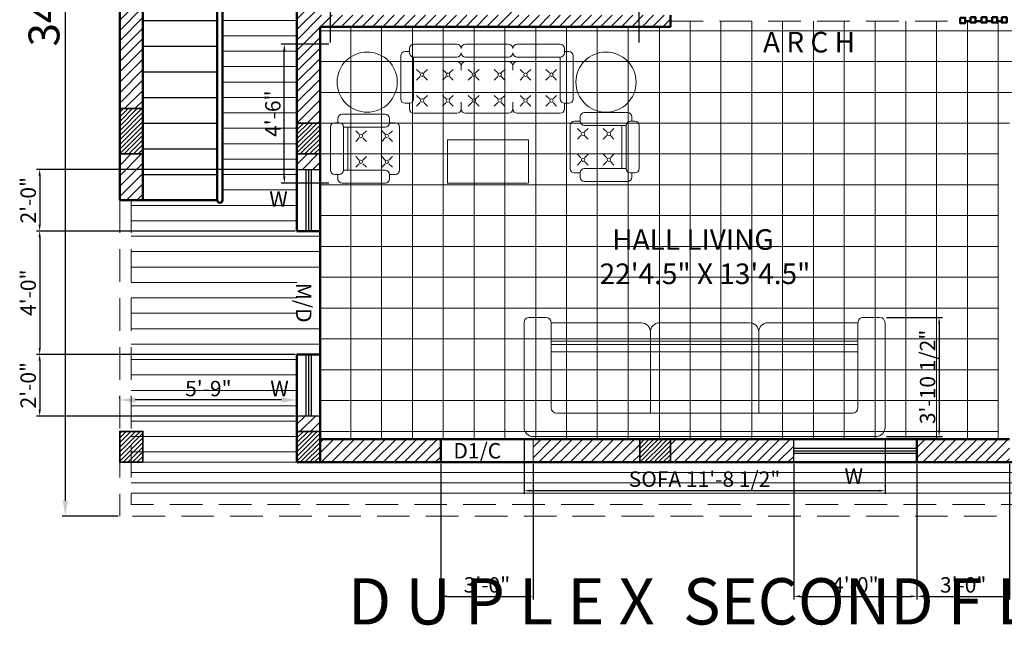
# Model space of a CAD drawing. Units: millimetres. Extents: x 225995 to 227247, y 225507 to 226008.
# Tile 1 of 23: x 225995 to 226378, y 225507 to 225743. Entities that reach past the tile are written whole.
import ezdxf

# ---------------------------------------------------------------- set-up
doc = ezdxf.new("R2010")
doc.units = ezdxf.units.MM
doc.linetypes.add('DASHED', pattern=[19.05, 12.7, -6.35])
for name, color, linetype, lineweight in [('A-ANNO-DIMS', 2, 'Continuous', 18), ('A-ANNO-TEXT', 3, 'Continuous', 18), ('A-AREA-IDEN', 30, 'Continuous', 18), ('A-COLS', 40, 'Continuous', 35), ('A-FLOR-PATT', 8, 'Continuous', 13), ('A-FLOR-STRS', 141, 'Continuous', 25), ('A-FURN', 9, 'Continuous', 18), ('A-GLAZ', 4, 'Continuous', 25), ('A-WALL', 7, 'Continuous', 50), ('A-WALL-OVHD', 1, 'DASHED', 18), ('A-WALL-PATT', 8, 'Continuous', 13)]:
    doc.layers.add(name, color=color, linetype=linetype, lineweight=lineweight)
doc.styles.get("Standard").update_dxf_attribs({"font": 'arial.ttf'})
doc.dimstyles.new('ISO-25', dxfattribs={"dimtxt": 6, "dimasz": 2.5, "dimexe": 1.25, "dimexo": 0.625, "dimtad": 1, "dimdec": 0, "dimlunit": 3, "dimtxsty": 'Standard', "dimcen": 2.5, "dimadec": 0, "dimazin": 0, "dimtfac": 1, "dimtdec": 0, "dimtmove": 0, "dimatfit": 3, "dimfxl": 1, "dimarcsym": 0})
pattern_1 = [(45, (-144, -120), (-0.898025612, 0.898025612), [])]

# ---------------------------------------------------------------- blocks, each defined once
blk = doc.blocks.new('A$C144B2C1F')
at = {"linetype": 'ByBlock'}
for p, q in [((1465, 1610), (965, 1610)), ((2065, 1610), (1565, 1610)), ((2665, 1610), (2165, 1610)), ((914, 1526), (864, 1526)), ((915, 1560), (915, 1510)), ((2764, 1526), (2714, 1526)), ((2715, 1510), (2715, 1560)), ((814, 1476), (814, 976)), ((964, 976), (964, 1460)), ((965, 1460), (1465, 1460)), ((965, 1410), (1465, 1410)), ((1565, 1460), (2065, 1460)), ((1565, 1410), (2065, 1410)), ((2165, 1460), (2665, 1460)), ((2165, 1410), (2664, 1410)), ((2664, 1460), (2664, 976)), ((2814, 976), (2814, 1476)), ((1040, 1277), (998, 1317)), ((1081, 1277), (1123, 1317)), ((1340, 1277), (1298, 1317)), ((1381, 1277), (1423, 1317)), ((1515, 1311), (1515, 1360)), ((1640, 1277), (1598, 1317)), ((1681, 1277), (1723, 1317)), ((1940, 1277), (1898, 1317)), ((1981, 1277), (2023, 1317)), ((2115, 1311), (2115, 1360)), ((2240, 1277), (2198, 1317)), ((2281, 1277), (2323, 1317)), ((2540, 1277), (2498, 1317)), ((2581, 1277), (2623, 1317)), ((1040, 1235), (998, 1193)), ((1081, 1235), (1123, 1193)), ((1340, 1235), (1298, 1193)), ((1381, 1235), (1423, 1193)), ((1640, 1235), (1598, 1193)), ((1681, 1235), (1723, 1193)), ((1940, 1235), (1898, 1193)), ((1981, 1235), (2023, 1193)), ((2240, 1235), (2198, 1193)), ((2281, 1235), (2323, 1193)), ((2540, 1235), (2498, 1193)), ((2581, 1235), (2623, 1193)), ((864, 926), (914, 926)), ((915, 926), (915, 860)), ((1040, 977), (998, 1017)), ((1040, 935), (998, 893)), ((1081, 977), (1123, 1017)), ((1081, 935), (1123, 893)), ((1340, 977), (1298, 1017)), ((1340, 935), (1298, 893)), ((1381, 977), (1423, 1017)), ((1381, 935), (1423, 893)), ((1515, 860), (1515, 937)), ((1515, 926), (1515, 860)), ((1640, 977), (1598, 1017)), ((1640, 935), (1598, 893)), ((1681, 977), (1723, 1017)), ((1681, 935), (1723, 893)), ((1940, 977), (1898, 1017)), ((1940, 935), (1898, 893)), ((1981, 977), (2023, 1017)), ((1981, 935), (2023, 893)), ((2115, 860), (2115, 937)), ((2115, 926), (2115, 860)), ((2240, 977), (2198, 1017)), ((2240, 935), (2198, 893)), ((2281, 977), (2323, 1017)), ((2281, 935), (2323, 893)), ((2540, 977), (2498, 1017)), ((2540, 935), (2498, 893)), ((2581, 977), (2623, 1017)), ((2581, 935), (2623, 893)), ((2714, 926), (2764, 926)), ((2715, 860), (2715, 926)), ((634, 800), (134, 800)), ((1129, 810), (965, 810)), ((1465, 810), (1088, 810)), ((1729, 810), (1565, 810)), ((2065, 810), (1688, 810)), ((2329, 810), (2165, 810)), ((2665, 810), (2288, 810)), ((3446, 819), (2946, 819)), ((100, 701), (50, 701)), ((84, 750), (84, 700)), ((684, 700), (684, 750)), ((750, 701), (684, 701)), ((2896, 718), (2830, 718)), ((2896, 769), (2896, 719)), ((3530, 718), (3480, 718)), ((3496, 719), (3496, 769)), ((0, 651), (0, 151)), ((150, 151), (150, 651)), ((150, 650), (634, 650)), ((200, 151), (200, 650)), ((333, 567), (293, 608)), ((375, 567), (418, 608)), ((633, 567), (593, 608)), ((675, 567), (718, 608)), ((800, 651), (800, 274)), ((2780, 504), (2780, 668)), ((2905, 593), (2863, 635)), ((2946, 669), (3430, 669)), ((2948, 593), (2987, 635)), ((3205, 593), (3163, 635)), ((3248, 593), (3287, 635)), ((3380, 668), (3380, 169)), ((3430, 668), (3430, 168)), ((3580, 168), (3580, 668)), ((333, 525), (293, 484)), ((375, 525), (418, 484)), ((633, 525), (593, 484)), ((675, 525), (718, 484)), ((2295, 501), (1355, 501)), ((1355, 501), (1355, 1)), ((2295, 1), (2295, 501)), ((2780, 168), (2780, 545)), ((2905, 552), (2863, 510)), ((2948, 552), (2987, 510)), ((3205, 552), (3163, 510)), ((3248, 552), (3287, 510)), ((333, 267), (293, 308)), ((375, 267), (418, 308)), ((633, 267), (593, 308)), ((675, 267), (718, 308)), ((800, 314), (800, 151)), ((2905, 293), (2863, 335)), ((2905, 252), (2863, 210)), ((2948, 293), (2987, 335)), ((2948, 252), (2987, 210)), ((3205, 293), (3163, 335)), ((3205, 252), (3163, 210)), ((3248, 293), (3287, 335)), ((3248, 252), (3287, 210)), ((634, 150), (150, 150)), ((333, 225), (293, 184)), ((375, 225), (418, 184)), ((633, 225), (593, 184)), ((675, 225), (718, 184)), ((2830, 118), (2896, 118)), ((2896, 119), (2896, 69)), ((3430, 169), (2946, 169)), ((3480, 118), (3530, 118)), ((3496, 69), (3496, 119)), ((50, 101), (100, 101)), ((84, 100), (84, 50)), ((134, 0), (634, 0)), ((684, 101), (750, 101)), ((684, 50), (684, 100)), ((1355, 1), (2285, 1)), ((2946, 19), (3446, 19))]:
    blk.add_line(p, q, dxfattribs=at)
for centre, radius in [((425, 1171), 349), ((3195, 1171), 349), ((1062, 1258), 20), ((1362, 1258), 20), ((1662, 1258), 20), ((1962, 1258), 20), ((2262, 1258), 20), ((2562, 1258), 20), ((1062, 958), 20), ((1362, 958), 20), ((1662, 958), 20), ((1962, 958), 20), ((2262, 958), 20), ((2562, 958), 20), ((2928, 571), 20), ((3228, 571), 20), ((352, 548), 20), ((652, 548), 20), ((352, 248), 20), ((652, 248), 20), ((2928, 271), 20), ((3228, 271), 20)]:
    blk.add_circle(centre, radius, dxfattribs=at)
for centre, start, end in [((965, 1560), 90, 180), ((965, 1560), 90, 180), ((1465, 1560), 0, 90), ((1565, 1560), 90, 180), ((1565, 1560), 90, 180), ((2065, 1560), 0, 90), ((2165, 1560), 90, 180), ((2165, 1560), 90, 180), ((2665, 1560), 0, 90), ((864, 1476), 90, 180), ((965, 1510), 180, 270), ((1465, 1510), 270, 0), ((1565, 1510), 180, 270), ((2065, 1510), 270, 0), ((2165, 1510), 180, 270), ((2665, 1510), 270, 0), ((2764, 1476), 0, 90), ((1465, 1360), 0, 90), ((1565, 1360), 90, 180), ((2065, 1360), 0, 90), ((2165, 1360), 90, 180), ((864, 976), 180, 270), ((914, 976), 270, 0), ((2714, 976), 180, 270), ((2764, 976), 270, 0), ((134, 750), 90, 180), ((634, 750), 0, 90), ((965, 860), 180, 270), ((1465, 860), 270, 0), ((1565, 860), 180, 270), ((2065, 860), 270, 0), ((2165, 860), 180, 270), ((2665, 860), 270, 0), ((2946, 769), 90, 180), ((3446, 769), 0, 90), ((50, 651), 90, 180), ((100, 651), 0, 90), ((634, 700), 270, 0), ((750, 651), 0, 90), ((2830, 668), 90, 180), ((2946, 719), 180, 270), ((3480, 668), 90, 180), ((3530, 668), 0, 90), ((3530, 668), 0, 90), ((50, 151), 180, 270), ((50, 151), 180, 270), ((100, 151), 270, 0), ((634, 100), 0, 90), ((750, 151), 270, 0), ((2830, 168), 180, 270), ((2946, 119), 90, 180), ((3480, 168), 180, 270), ((3530, 168), 270, 0), ((134, 50), 180, 270), ((634, 50), 270, 0), ((2946, 69), 180, 270), ((3446, 69), 270, 0)]:
    blk.add_arc(centre, 50, start, end, dxfattribs=at)
blk = doc.blocks.new('A$C05BA3A2B')
for p, q in [((0.05, 0.6596), (1.95, 0.6596)), ((0.05, 0.6596), (1.95, 0.6596)), ((0.05, 0.6596), (1.95, 0.6596)), ((0, 0.03), (0, 0.6096)), ((0, 0.03), (0, 0.6096)), ((0, 0.03), (0, 0.6096)), ((2, 0.6096), (2, 0.03)), ((2, 0.6096), (2, 0.03)), ((2, 0.6096), (2, 0.03)), ((0.15, 0.5), (0.15, 0.03)), ((0.15, 0.5), (0.15, 0.03)), ((0.15, 0.5), (0.15, 0.03)), ((1.82, 0.53), (0.18, 0.53)), ((1.82, 0.53), (0.18, 0.53)), ((1.82, 0.53), (0.18, 0.53)), ((0.7, 0.08), (0.7, 0.53)), ((0.7, 0.08), (0.7, 0.53)), ((0.7, 0.08), (0.7, 0.53)), ((1.3, 0.53), (1.3, 0.08)), ((1.3, 0.53), (1.3, 0.08)), ((1.3, 0.53), (1.3, 0.08)), ((1.85, 0.03), (1.85, 0.5)), ((1.85, 0.03), (1.85, 0.5)), ((1.85, 0.03), (1.85, 0.5)), ((1.85, 0.1908), (0.15, 0.1908)), ((1.85, 0.1908), (0.15, 0.1908)), ((1.85, 0.1908), (0.15, 0.1908)), ((1.85, 0.1508), (0.15, 0.1508)), ((1.85, 0.1508), (0.15, 0.1508)), ((1.85, 0.1508), (0.15, 0.1508)), ((1.85, 0.1308), (0.15, 0.1308)), ((1.85, 0.1308), (0.15, 0.1308)), ((1.85, 0.1308), (0.15, 0.1308)), ((0.12, 0), (0.03, 0)), ((0.12, 0), (0.03, 0)), ((0.12, 0), (0.03, 0)), ((0.65, 0.03), (0.15, 0.03)), ((0.65, 0.03), (0.15, 0.03)), ((0.65, 0.03), (0.15, 0.03)), ((1.25, 0.03), (0.75, 0.03)), ((1.25, 0.03), (0.75, 0.03)), ((1.25, 0.03), (0.75, 0.03)), ((1.85, 0.03), (1.35, 0.03)), ((1.85, 0.03), (1.35, 0.03)), ((1.85, 0.03), (1.35, 0.03)), ((1.97, 0), (1.88, 0)), ((1.97, 0), (1.88, 0)), ((1.97, 0), (1.88, 0))]:
    blk.add_line(p, q)
for centre, radius, start, end in [((0.05, 0.6096), 0.05, 90, 180), ((0.05, 0.6096), 0.05, 90, 180), ((0.05, 0.6096), 0.05, 90, 180), ((1.95, 0.6096), 0.05, 0, 90), ((1.95, 0.6096), 0.05, 0, 90), ((1.95, 0.6096), 0.05, 0, 90), ((0.18, 0.5), 0.03, 90, 180), ((0.18, 0.5), 0.03, 90, 180), ((0.18, 0.5), 0.03, 90, 180), ((1.82, 0.5), 0.03, 0, 90), ((1.82, 0.5), 0.03, 0, 90), ((1.82, 0.5), 0.03, 0, 90), ((0.65, 0.08), 0.05, 270, 0), ((0.65, 0.08), 0.05, 270, 0), ((0.65, 0.08), 0.05, 270, 0), ((0.75, 0.08), 0.05, 180, 270), ((0.75, 0.08), 0.05, 180, 270), ((0.75, 0.08), 0.05, 180, 270), ((1.25, 0.08), 0.05, 270, 0), ((1.25, 0.08), 0.05, 270, 0), ((1.25, 0.08), 0.05, 270, 0), ((1.35, 0.08), 0.05, 180, 270), ((1.35, 0.08), 0.05, 180, 270), ((1.35, 0.08), 0.05, 180, 270), ((0.03, 0.03), 0.03, 180, 270), ((0.03, 0.03), 0.03, 180, 270), ((0.03, 0.03), 0.03, 180, 270), ((0.12, 0.03), 0.03, 270, 0), ((0.12, 0.03), 0.03, 270, 0), ((0.12, 0.03), 0.03, 270, 0), ((1.88, 0.03), 0.03, 180, 270), ((1.88, 0.03), 0.03, 180, 270), ((1.88, 0.03), 0.03, 180, 270), ((1.97, 0.03), 0.03, 270, 0), ((1.97, 0.03), 0.03, 270, 0), ((1.97, 0.03), 0.03, 270, 0)]:
    blk.add_arc(centre, radius, start, end)
blk = doc.blocks.new('A$C720744B6')
blk.add_blockref('A$C05BA3A2B', (0, 0))
blk = doc.blocks.new('*D66')
at = {"layer": 'A-ANNO-DIMS', "color": 0, "lineweight": -2, "transparency": 16777216}
for p, q in [((226033.88, 225595.63), (226033.88, 225596.26)), ((226096.88, 225595.01), (226039.88, 225595.01)), ((226102.88, 225595.63), (226102.88, 225596.26))]:
    blk.add_line(p, q, dxfattribs=at)
at = {"layer": 'A-ANNO-DIMS', "color": 0, "transparency": 16777216}
for points in [[(226039.88, 225596.01), (226039.88, 225594.01), (226033.88, 225595.01)], [(226096.88, 225596.01), (226096.88, 225594.01), (226102.88, 225595.01)]]:
    blk.add_solid(points, dxfattribs=at)
at = {"layer": 'Defpoints', "color": 0, "transparency": 16777216}
for p in [(226033.88, 225595.01), (226033.88, 225595.01), (226102.88, 225595.01)]:
    blk.add_point(p, dxfattribs=at)
at = {"layer": 'A-ANNO-DIMS', "color": 0, "transparency": 16777216, "insert": (226068.38, 225598.69), "char_height": 6, "attachment_point": 5}
blk.add_mtext('5\'-9"', dxfattribs=at)
blk = doc.blocks.new('*D69')
at = {"layer": 'A-ANNO-DIMS', "color": 0, "lineweight": -2, "transparency": 16777216}
for p, q in [((226033.25, 225960.77), (226011.42, 225960.77)), ((226012.67, 225954.77), (226012.67, 225555.77)), ((226033.25, 225549.77), (226011.42, 225549.77))]:
    blk.add_line(p, q, dxfattribs=at)
at = {"layer": 'A-ANNO-DIMS', "color": 0, "transparency": 16777216}
for points in [[(226011.67, 225954.77), (226013.67, 225954.77), (226012.67, 225960.77)], [(226011.67, 225555.77), (226013.67, 225555.77), (226012.67, 225549.77)]]:
    blk.add_solid(points, dxfattribs=at)
at = {"layer": 'Defpoints', "color": 0, "transparency": 16777216}
for p in [(226033.88, 225960.77), (226012.67, 225549.77), (226033.88, 225549.77)]:
    blk.add_point(p, dxfattribs=at)
at = {"layer": 'A-ANNO-DIMS', "color": 0, "transparency": 16777216, "insert": (226005.92, 225755.27), "char_height": 12, "attachment_point": 5, "rotation": 90}
blk.add_mtext('34\'-3"', dxfattribs=at)
blk = doc.blocks.new('*D83')
at = {"layer": 'A-ANNO-DIMS', "color": 0, "lineweight": -2, "transparency": 16777216}
for p, q in [((226115.99, 225734.11), (226115.99, 225752.77)), ((226118.49, 225751.52), (226233.69, 225751.52)), ((226236.19, 225734.11), (226236.19, 225752.77))]:
    blk.add_line(p, q, dxfattribs=at)
at = {"layer": 'A-ANNO-DIMS', "color": 0, "transparency": 16777216}
for points in [[(226118.49, 225751.93), (226118.49, 225751.1), (226115.99, 225751.52)], [(226233.69, 225751.93), (226233.69, 225751.1), (226236.19, 225751.52)]]:
    blk.add_solid(points, dxfattribs=at)
at = {"layer": 'Defpoints', "color": 0, "transparency": 16777216}
for p in [(226236.19, 225751.52), (226115.99, 225733.49), (226236.19, 225733.49)]:
    blk.add_point(p, dxfattribs=at)
at = {"layer": 'A-ANNO-DIMS', "color": 0, "transparency": 16777216, "insert": (226176.09, 225755.25), "char_height": 6, "attachment_point": 5}
blk.add_mtext('SOFA SET 10\'-0"', dxfattribs=at)
blk = doc.blocks.new('*D84')
at = {"layer": 'A-ANNO-DIMS', "color": 0, "lineweight": -2, "transparency": 16777216}
for p, q in [((226115.37, 225733.49), (226096.71, 225733.49)), ((226097.96, 225681.93), (226097.96, 225730.99)), ((226115.37, 225679.43), (226096.71, 225679.43))]:
    blk.add_line(p, q, dxfattribs=at)
at = {"layer": 'A-ANNO-DIMS', "color": 0, "transparency": 16777216}
for points in [[(226097.54, 225730.99), (226098.38, 225730.99), (226097.96, 225733.49)], [(226097.54, 225681.93), (226098.38, 225681.93), (226097.96, 225679.43)]]:
    blk.add_solid(points, dxfattribs=at)
at = {"layer": 'Defpoints', "color": 0, "transparency": 16777216}
for p in [(226097.96, 225733.49), (226115.99, 225733.49), (226115.99, 225679.43)]:
    blk.add_point(p, dxfattribs=at)
at = {"layer": 'A-ANNO-DIMS', "color": 0, "transparency": 16777216, "insert": (226094.27, 225706.46), "char_height": 6, "attachment_point": 5, "rotation": 90}
blk.add_mtext('4\'-6"', dxfattribs=at)
blk = doc.blocks.new('*D85')
at = {"layer": 'A-ANNO-DIMS', "color": 0, "lineweight": -2, "transparency": 16777216}
for p, q in [((226191.34, 225580.17), (226191.34, 225558.45)), ((226331.94, 225580.17), (226331.94, 225558.45)), ((226329.44, 225559.7), (226193.84, 225559.7))]:
    blk.add_line(p, q, dxfattribs=at)
at = {"layer": 'A-ANNO-DIMS', "color": 0, "transparency": 16777216}
for points in [[(226193.84, 225560.12), (226193.84, 225559.29), (226191.34, 225559.7)], [(226329.44, 225560.12), (226329.44, 225559.29), (226331.94, 225559.7)]]:
    blk.add_solid(points, dxfattribs=at)
at = {"layer": 'Defpoints', "color": 0, "transparency": 16777216}
for p in [(226191.34, 225580.79), (226331.94, 225580.79), (226191.34, 225559.7)]:
    blk.add_point(p, dxfattribs=at)
at = {"layer": 'A-ANNO-DIMS', "color": 0, "transparency": 16777216, "insert": (226261.64, 225563.43), "char_height": 6, "attachment_point": 5}
blk.add_mtext('SOFA 11\'-8 1/2"', dxfattribs=at)
blk = doc.blocks.new('*D86')
at = {"layer": 'A-ANNO-DIMS', "color": 0, "lineweight": -2, "transparency": 16777216}
for p, q in [((226332.56, 225627.16), (226354.27, 225627.16)), ((226353.02, 225624.66), (226353.02, 225583.29)), ((226332.56, 225580.79), (226354.27, 225580.79))]:
    blk.add_line(p, q, dxfattribs=at)
at = {"layer": 'A-ANNO-DIMS', "color": 0, "transparency": 16777216}
for points in [[(226352.61, 225624.66), (226353.44, 225624.66), (226353.02, 225627.16)], [(226352.61, 225583.29), (226353.44, 225583.29), (226353.02, 225580.79)]]:
    blk.add_solid(points, dxfattribs=at)
at = {"layer": 'Defpoints', "color": 0, "transparency": 16777216}
for p in [(226331.94, 225627.16), (226331.94, 225580.79), (226353.02, 225580.79)]:
    blk.add_point(p, dxfattribs=at)
at = {"layer": 'A-ANNO-DIMS', "color": 0, "transparency": 16777216, "insert": (226349.3, 225603.98), "char_height": 6, "attachment_point": 5, "rotation": 90}
blk.add_mtext('3\'-10 1/2"', dxfattribs=at)
blk = doc.blocks.new('*D106')
at = {"layer": 'A-ANNO-DIMS', "color": 0, "lineweight": -2, "transparency": 16777216}
for p, q in [((226296.38, 225570.15), (226296.38, 225517.32)), ((226344.38, 225570.15), (226344.38, 225517.32)), ((226298.88, 225518.57), (226341.88, 225518.57))]:
    blk.add_line(p, q, dxfattribs=at)
at = {"layer": 'A-ANNO-DIMS', "color": 0, "transparency": 16777216}
for points in [[(226298.88, 225518.99), (226298.88, 225518.16), (226296.38, 225518.57)], [(226341.88, 225518.99), (226341.88, 225518.16), (226344.38, 225518.57)]]:
    blk.add_solid(points, dxfattribs=at)
at = {"layer": 'Defpoints', "color": 0, "transparency": 16777216}
for p in [(226296.38, 225570.77), (226344.38, 225570.77), (226344.38, 225518.57)]:
    blk.add_point(p, dxfattribs=at)
at = {"layer": 'A-ANNO-DIMS', "color": 0, "transparency": 16777216, "insert": (226320.38, 225522.26), "char_height": 6, "attachment_point": 5}
blk.add_mtext('4\'-0"', dxfattribs=at)
blk = doc.blocks.new('*D107')
at = {"layer": 'A-ANNO-DIMS', "color": 0, "lineweight": -2, "transparency": 16777216}
for p, q in [((226344.38, 225570.15), (226344.38, 225517.32)), ((226380.38, 225570.15), (226380.38, 225517.32)), ((226346.88, 225518.57), (226377.88, 225518.57))]:
    blk.add_line(p, q, dxfattribs=at)
at = {"layer": 'A-ANNO-DIMS', "color": 0, "transparency": 16777216}
for points in [[(226346.88, 225518.99), (226346.88, 225518.16), (226344.38, 225518.57)], [(226377.88, 225518.99), (226377.88, 225518.16), (226380.38, 225518.57)]]:
    blk.add_solid(points, dxfattribs=at)
at = {"layer": 'Defpoints', "color": 0, "transparency": 16777216}
for p in [(226344.38, 225570.77), (226380.38, 225570.77), (226380.38, 225518.57)]:
    blk.add_point(p, dxfattribs=at)
at = {"layer": 'A-ANNO-DIMS', "color": 0, "transparency": 16777216, "insert": (226362.38, 225522.26), "char_height": 6, "attachment_point": 5}
blk.add_mtext('3\'-0"', dxfattribs=at)
blk = doc.blocks.new('*D108')
at = {"layer": 'A-ANNO-DIMS', "color": 0, "lineweight": -2, "transparency": 16777216}
for p, q in [((226158.88, 225570.15), (226158.88, 225517.32)), ((226194.88, 225570.15), (226194.88, 225517.32)), ((226161.38, 225518.57), (226192.38, 225518.57))]:
    blk.add_line(p, q, dxfattribs=at)
at = {"layer": 'A-ANNO-DIMS', "color": 0, "transparency": 16777216}
for points in [[(226161.38, 225518.99), (226161.38, 225518.16), (226158.88, 225518.57)], [(226192.38, 225518.99), (226192.38, 225518.16), (226194.88, 225518.57)]]:
    blk.add_solid(points, dxfattribs=at)
at = {"layer": 'Defpoints', "color": 0, "transparency": 16777216}
for p in [(226158.88, 225570.77), (226194.88, 225570.77), (226194.88, 225518.57)]:
    blk.add_point(p, dxfattribs=at)
at = {"layer": 'A-ANNO-DIMS', "color": 0, "transparency": 16777216, "insert": (226176.88, 225522.26), "char_height": 6, "attachment_point": 5}
blk.add_mtext('3\'-0"', dxfattribs=at)
blk = doc.blocks.new('*D109')
at = {"layer": 'A-ANNO-DIMS', "color": 0, "lineweight": -2, "transparency": 16777216}
for p, q in [((226102.25, 225684.77), (226001.43, 225684.77)), ((226002.68, 225682.27), (226002.68, 225663.27)), ((226102.25, 225660.77), (226001.43, 225660.77))]:
    blk.add_line(p, q, dxfattribs=at)
at = {"layer": 'A-ANNO-DIMS', "color": 0, "transparency": 16777216}
for points in [[(226002.26, 225682.27), (226003.09, 225682.27), (226002.68, 225684.77)], [(226002.26, 225663.27), (226003.09, 225663.27), (226002.68, 225660.77)]]:
    blk.add_solid(points, dxfattribs=at)
at = {"layer": 'Defpoints', "color": 0, "transparency": 16777216}
for p in [(226102.88, 225684.77), (226002.68, 225660.77), (226102.88, 225660.77)]:
    blk.add_point(p, dxfattribs=at)
at = {"layer": 'A-ANNO-DIMS', "color": 0, "transparency": 16777216, "insert": (225998.99, 225672.77), "char_height": 6, "attachment_point": 5, "rotation": 90}
blk.add_mtext('2\'-0"', dxfattribs=at)
blk = doc.blocks.new('*D110')
at = {"layer": 'A-ANNO-DIMS', "color": 0, "lineweight": -2, "transparency": 16777216}
for p, q in [((226102.25, 225660.77), (226001.43, 225660.77)), ((226002.68, 225658.27), (226002.68, 225615.27)), ((226102.25, 225612.77), (226001.43, 225612.77))]:
    blk.add_line(p, q, dxfattribs=at)
at = {"layer": 'A-ANNO-DIMS', "color": 0, "transparency": 16777216}
for points in [[(226002.26, 225658.27), (226003.09, 225658.27), (226002.68, 225660.77)], [(226002.26, 225615.27), (226003.09, 225615.27), (226002.68, 225612.77)]]:
    blk.add_solid(points, dxfattribs=at)
at = {"layer": 'Defpoints', "color": 0, "transparency": 16777216}
for p in [(226102.88, 225660.77), (226002.68, 225612.77), (226102.88, 225612.77)]:
    blk.add_point(p, dxfattribs=at)
at = {"layer": 'A-ANNO-DIMS', "color": 0, "transparency": 16777216, "insert": (225998.99, 225636.77), "char_height": 6, "attachment_point": 5, "rotation": 90}
blk.add_mtext('4\'-0"', dxfattribs=at)
blk = doc.blocks.new('*D111')
at = {"layer": 'A-ANNO-DIMS', "color": 0, "lineweight": -2, "transparency": 16777216}
for p, q in [((226102.25, 225612.77), (226001.43, 225612.77)), ((226002.68, 225610.27), (226002.68, 225591.27)), ((226102.25, 225588.77), (226001.43, 225588.77))]:
    blk.add_line(p, q, dxfattribs=at)
at = {"layer": 'A-ANNO-DIMS', "color": 0, "transparency": 16777216}
for points in [[(226002.26, 225610.27), (226003.09, 225610.27), (226002.68, 225612.77)], [(226002.26, 225591.27), (226003.09, 225591.27), (226002.68, 225588.77)]]:
    blk.add_solid(points, dxfattribs=at)
at = {"layer": 'Defpoints', "color": 0, "transparency": 16777216}
for p in [(226102.88, 225612.77), (226002.68, 225588.77), (226102.88, 225588.77)]:
    blk.add_point(p, dxfattribs=at)
at = {"layer": 'A-ANNO-DIMS', "color": 0, "transparency": 16777216, "insert": (225998.99, 225600.77), "char_height": 6, "attachment_point": 5, "rotation": 90}
blk.add_mtext('2\'-0"', dxfattribs=at)

msp = doc.modelspace()

# ---------------------------------------------------------------- hatches: boundary and pattern name
at = {"layer": 'A-WALL-PATT'}
h = msp.add_hatch(dxfattribs=at)
h.set_pattern_fill('ANSI31', color=256, scale=0.9)
h.paths.add_polyline_path([(226042.88, 225894.68), (226033.88, 225894.68), (226033.88, 225708.42), (226042.88, 225708.42)])
h = msp.add_hatch(dxfattribs=at)
h.set_pattern_fill('ANSI31', color=256, scale=0.9)
h.paths.add_polyline_path([(226111.88, 225740.27), (226248.38, 225740.27), (226248.38, 225744.77), (226188.38, 225744.77), (226188.38, 225756.77), (226183.88, 225756.77), (226183.88, 225744.77), (226111.88, 225744.77), (226111.88, 225762.77), (226102.88, 225762.77), (226102.88, 225702.77), (226111.88, 225702.77)])
h = msp.add_hatch(dxfattribs=at)
h.set_pattern_fill('ANSI31', color=256, scale=0.4)
h.paths.add_polyline_path([(226042.88, 225708.42), (226033.88, 225708.42), (226033.88, 225690.77), (226042.88, 225690.77)])
h = msp.add_hatch(dxfattribs=at)
h.set_pattern_fill('ANSI31', color=256, scale=0.4)
h.set_pattern_definition([(45, (-3e-11, 120), (-0.898025612, 0.898025612), [])])
h.paths.add_polyline_path([(226111.88, 225702.77), (226102.88, 225702.77), (226102.88, 225690.77), (226111.88, 225690.77)])
h = msp.add_hatch(dxfattribs=at)
h.set_pattern_fill('ANSI31', color=256, scale=0.9)
h.paths.add_polyline_path([(226042.88, 225690.77), (226033.88, 225690.77), (226033.88, 225672.77), (226042.88, 225672.77)])
h = msp.add_hatch(dxfattribs=at)
h.set_pattern_fill('ANSI31', color=256, scale=0.9)
h.paths.add_polyline_path([(226111.88, 225690.77), (226102.88, 225690.77), (226102.88, 225684.77), (226111.88, 225684.77)])
h = msp.add_hatch(dxfattribs=at)
h.set_pattern_fill('ANSI31', color=256, scale=0.9)
h.paths.add_polyline_path([(226111.88, 225588.77), (226102.88, 225588.77), (226102.88, 225582.77), (226111.88, 225582.77)])
h = msp.add_hatch(dxfattribs=at)
h.set_pattern_fill('ANSI31', color=256, scale=0.4)
h.set_pattern_definition([(45, (-69, 0), (-0.898025612, 0.898025612), [])])
h.paths.add_polyline_path([(226042.88, 225582.77), (226033.88, 225582.77), (226033.88, 225570.77), (226042.88, 225570.77)])
h = msp.add_hatch(dxfattribs=at)
h.set_pattern_fill('ANSI31', color=256, scale=0.4)
h.paths.add_polyline_path([(226111.88, 225582.77), (226102.88, 225582.77), (226102.88, 225570.77), (226111.88, 225570.77)])
h = msp.add_hatch(dxfattribs=at)
h.set_pattern_fill('ANSI31', color=256, scale=0.9)
h.paths.add_polyline_path([(226158.88, 225579.77), (226111.88, 225579.77), (226111.88, 225570.77), (226158.88, 225570.77)])
h = msp.add_hatch(dxfattribs=at)
h.set_pattern_fill('ANSI31', color=256, scale=0.9)
h.paths.add_polyline_path([(226236.38, 225579.77), (226194.88, 225579.77), (226194.88, 225570.77), (226236.38, 225570.77)])
h = msp.add_hatch(dxfattribs=at)
h.set_pattern_fill('ANSI31', color=256, scale=0.4)
h.set_pattern_definition(pattern_1)
h.paths.add_polyline_path([(226240.88, 225579.77), (226236.38, 225579.77), (226236.38, 225575.27), (226240.88, 225575.27)])
h = msp.add_hatch(dxfattribs=at)
h.set_pattern_fill('ANSI31', color=256, scale=0.4)
h.set_pattern_definition(pattern_1)
h.paths.add_polyline_path([(226248.38, 225579.77), (226240.88, 225579.77), (226240.88, 225575.27), (226248.38, 225575.27)])
h = msp.add_hatch(dxfattribs=at)
h.set_pattern_fill('ANSI31', color=256, scale=0.9)
h.paths.add_polyline_path([(226296.38, 225579.77), (226248.38, 225579.77), (226248.38, 225570.77), (226296.38, 225570.77)])
h = msp.add_hatch(dxfattribs=at)
h.set_pattern_fill('ANSI31', color=256, scale=0.9)
h.paths.add_polyline_path([(226380.38, 225579.77), (226344.38, 225579.77), (226344.38, 225570.77), (226380.38, 225570.77)])
h = msp.add_hatch(dxfattribs=at)
h.set_pattern_fill('ANSI31', color=256, scale=0.4)
h.set_pattern_definition(pattern_1)
h.paths.add_polyline_path([(226240.88, 225575.27), (226236.38, 225575.27), (226236.38, 225570.77), (226240.88, 225570.77)])
h = msp.add_hatch(dxfattribs=at)
h.set_pattern_fill('ANSI31', color=256, scale=0.4)
h.set_pattern_definition(pattern_1)
h.paths.add_polyline_path([(226248.38, 225575.27), (226240.88, 225575.27), (226240.88, 225570.77), (226248.38, 225570.77)])

# ---------------------------------------------------------------- linework, layer by layer
at = {"layer": 'A-COLS'}
for points in [[(226042.88, 225690.77), (226033.88, 225690.77), (226033.88, 225708.42), (226042.88, 225708.42)], [(226111.88, 225690.77), (226102.88, 225690.77), (226102.88, 225702.77), (226111.88, 225702.77)], [(226042.88, 225570.77), (226033.88, 225570.77), (226033.88, 225582.77), (226042.88, 225582.77)], [(226111.88, 225570.77), (226102.88, 225570.77), (226102.88, 225582.77), (226111.88, 225582.77)], [(226236.38, 225570.77), (226236.38, 225579.77), (226248.38, 225579.77), (226248.38, 225570.77)]]:
    msp.add_lwpolyline(points, close=True, dxfattribs=at)
at = {"layer": 'A-FLOR-PATT'}
for p, q in [((226102.88, 225742.77), (226073.88, 225742.77)), ((226123.88, 225579.77), (226123.88, 225740.27)), ((226135.88, 225579.77), (226135.88, 225740.27)), ((226147.88, 225579.77), (226147.88, 225740.27)), ((226159.88, 225579.77), (226159.88, 225740.27)), ((226171.88, 225579.77), (226171.88, 225740.27)), ((226183.88, 225579.77), (226183.88, 225740.27)), ((226195.88, 225579.77), (226195.88, 225740.27)), ((226207.88, 225579.77), (226207.88, 225740.27)), ((226219.88, 225579.77), (226219.88, 225740.27)), ((226231.88, 225579.77), (226231.88, 225740.27)), ((226244.05, 225740.27), (226244.05, 225579.77)), ((226256.05, 225742.52), (226256.05, 225579.77)), ((226268.05, 225742.52), (226268.05, 225579.77)), ((226280.05, 225742.52), (226280.05, 225579.77)), ((226292.05, 225742.52), (226292.05, 225579.77)), ((226304.05, 225742.52), (226304.05, 225579.77)), ((226316.05, 225742.52), (226316.05, 225579.77)), ((226328.05, 225742.52), (226328.05, 225579.77)), ((226340.05, 225742.52), (226340.05, 225579.77)), ((226352.05, 225742.52), (226352.05, 225579.77)), ((226364.05, 225742.52), (226364.05, 225579.77)), ((226376.05, 225742.52), (226376.05, 225579.77)), ((226102.88, 225736.77), (226073.88, 225736.77)), ((226111.88, 225738.77), (226557.38, 225738.77)), ((226102.88, 225730.77), (226073.88, 225730.77)), ((226102.88, 225724.77), (226073.88, 225724.77)), ((226111.88, 225726.77), (226557.38, 225726.77)), ((226102.88, 225718.77), (226073.88, 225718.77)), ((226111.88, 225714.77), (226557.38, 225714.77)), ((226102.88, 225712.77), (226073.88, 225712.77)), ((226102.88, 225706.77), (226073.88, 225706.77)), ((226111.88, 225702.77), (226380.38, 225702.77)), ((226102.88, 225700.77), (226073.88, 225700.77)), ((226102.88, 225694.77), (226073.88, 225694.77)), ((226111.88, 225690.77), (226376.05, 225690.77)), ((226102.88, 225688.77), (226073.88, 225688.77)), ((226102.88, 225682.77), (226073.88, 225682.77)), ((226111.88, 225678.77), (226376.05, 225678.77)), ((226102.88, 225676.77), (226073.88, 225676.77)), ((226102.88, 225670.77), (226038.38, 225670.77)), ((226102.88, 225664.77), (226038.38, 225664.77)), ((226111.88, 225666.77), (226376.05, 225666.77)), ((226111.88, 225658.77), (226038.38, 225658.77)), ((226111.88, 225652.77), (226038.38, 225652.77)), ((226111.88, 225654.77), (226376.05, 225654.77)), ((226111.88, 225646.77), (226038.38, 225646.77)), ((226102.88, 225640.77), (226038.38, 225640.77)), ((226111.88, 225642.77), (226376.05, 225642.77)), ((226102.88, 225634.77), (226038.38, 225634.77)), ((226111.88, 225630.77), (226376.05, 225630.77)), ((226102.88, 225628.77), (226038.38, 225628.77)), ((226111.88, 225622.77), (226038.38, 225622.77)), ((226111.88, 225618.77), (226376.05, 225618.77)), ((226111.88, 225616.77), (226038.38, 225616.77)), ((226102.88, 225610.77), (226038.38, 225610.77)), ((226111.88, 225606.77), (226376.05, 225606.77)), ((226102.88, 225604.77), (226038.38, 225604.77)), ((226102.88, 225598.77), (226038.38, 225598.77)), ((226111.88, 225594.77), (226376.05, 225594.77)), ((226102.88, 225592.77), (226038.38, 225592.77)), ((226102.88, 225586.77), (226038.38, 225586.77)), ((226111.88, 225582.77), (226376.05, 225582.77)), ((226102.88, 225580.77), (226038.38, 225580.77)), ((226102.88, 225574.77), (226038.38, 225574.77)), ((226102.88, 225570.77), (226038.38, 225570.77)), ((226038.38, 225566.77), (226561.38, 225566.77)), ((226038.38, 225562.77), (226561.38, 225562.77)), ((226038.38, 225558.77), (226561.38, 225558.77))]:
    msp.add_line(p, q, dxfattribs=at)
at = {"layer": 'A-FLOR-STRS'}
for p, q in [((226042.88, 225742.77), (226071.88, 225742.77)), ((226042.88, 225732.77), (226071.88, 225732.77)), ((226042.88, 225722.77), (226071.88, 225722.77)), ((226042.88, 225712.77), (226071.88, 225712.77)), ((226042.88, 225702.77), (226071.88, 225702.77)), ((226042.88, 225692.77), (226071.88, 225692.77)), ((226042.88, 225682.77), (226071.88, 225682.77))]:
    msp.add_line(p, q, dxfattribs=at)
at = {"layer": 'A-FURN'}
for p, q in [((226111.88, 225588.77), (226102.88, 225588.77)), ((226042.88, 225579.77), (226042.88, 225570.77)), ((226194.88, 225579.77), (226194.88, 225570.77)), ((226194.88, 225579.77), (226296.38, 225579.77)), ((226236.38, 225579.77), (226236.38, 225570.77)), ((226248.38, 225579.77), (226248.38, 225570.77)), ((226296.38, 225579.77), (226296.38, 225570.77)), ((226194.88, 225570.77), (226296.38, 225570.77)), ((226243.88, 225570.79), (226248.38, 225570.77))]:
    msp.add_line(p, q, dxfattribs=at)
at = {"layer": 'A-GLAZ'}
for p, q in [((226106.38, 225684.77), (226106.38, 225660.77)), ((226107.38, 225684.77), (226107.38, 225660.77)), ((226108.38, 225684.77), (226108.38, 225660.77)), ((226106.38, 225612.77), (226106.38, 225588.77)), ((226107.38, 225612.77), (226107.38, 225588.77)), ((226108.38, 225612.77), (226108.38, 225588.77)), ((226296.38, 225576.27), (226344.38, 225576.27)), ((226296.38, 225575.27), (226344.38, 225575.27)), ((226296.38, 225574.27), (226344.38, 225574.27))]:
    msp.add_line(p, q, dxfattribs=at)
for points in [[(226102.88, 225684.77), (226111.88, 225684.77), (226111.88, 225660.77), (226102.88, 225660.77)], [(226102.88, 225612.77), (226111.88, 225612.77), (226111.88, 225588.77), (226102.88, 225588.77)], [(226296.38, 225579.77), (226344.38, 225579.77), (226344.38, 225570.77), (226296.38, 225570.77)]]:
    msp.add_lwpolyline(points, close=True, dxfattribs=at)
at = {"layer": 'A-WALL'}
for p, q in [((226033.88, 225672.77), (226033.88, 225960.77)), ((226033.88, 225960.77), (226033.88, 225672.77)), ((226042.88, 225672.77), (226042.88, 225951.77)), ((226042.88, 225672.77), (226042.88, 225894.77)), ((226102.88, 225660.77), (226102.88, 225894.77)), ((226102.88, 225894.77), (226102.88, 225660.77)), ((226071.88, 225852.77), (226071.88, 225672.77)), ((226073.88, 225852.77), (226073.88, 225672.77)), ((226248.38, 225740.27), (226248.38, 225744.77)), ((226248.38, 225740.27), (226248.38, 225744.77)), ((226111.88, 225740.27), (226248.38, 225740.27)), ((226111.88, 225660.77), (226111.88, 225740.27)), ((226111.88, 225660.77), (226111.88, 225740.27)), ((226111.88, 225740.27), (226248.38, 225740.27)), ((226363.18, 225742.52), (226365.24, 225742.52)), ((226367.21, 225742.52), (226369.52, 225742.52)), ((226371.49, 225742.52), (226373.67, 225742.52)), ((226375.64, 225742.52), (226377.42, 225742.52)), ((226042.88, 225672.77), (226033.88, 225672.77)), ((226033.88, 225672.77), (226042.88, 225672.77)), ((226042.88, 225672.77), (226071.88, 225672.77)), ((226102.88, 225660.77), (226111.88, 225660.77)), ((226102.88, 225660.77), (226111.88, 225660.77)), ((226111.88, 225660.77), (226111.88, 225612.77)), ((226111.88, 225660.77), (226111.88, 225612.77)), ((226102.88, 225570.77), (226102.88, 225612.77)), ((226111.88, 225612.77), (226102.88, 225612.77)), ((226111.88, 225612.77), (226102.88, 225612.77)), ((226102.88, 225612.77), (226102.88, 225570.77)), ((226111.88, 225579.77), (226111.88, 225612.77)), ((226111.88, 225579.77), (226111.88, 225612.77)), ((226111.88, 225579.77), (226158.88, 225579.77)), ((226111.88, 225579.77), (226111.88, 225570.77)), ((226380.38, 225579.77), (226111.88, 225579.77)), ((226158.88, 225579.77), (226158.88, 225570.77)), ((226344.38, 225579.77), (226344.38, 225570.77)), ((226344.38, 225579.77), (226380.38, 225579.77)), ((226102.88, 225570.77), (226158.88, 225570.77)), ((226102.88, 225570.77), (226565.88, 225570.77)), ((226344.38, 225570.77), (226565.88, 225570.77))]:
    msp.add_line(p, q, dxfattribs=at)
for points in [[(226365.24, 225743.99), (226367.21, 225743.99), (226367.21, 225741.91), (226365.24, 225741.91)], [(226369.52, 225743.99), (226371.49, 225743.99), (226371.49, 225741.91), (226369.52, 225741.91)], [(226373.67, 225743.99), (226375.64, 225743.99), (226375.64, 225741.91), (226373.67, 225741.91)], [(226377.42, 225743.99), (226379.39, 225743.99), (226379.39, 225741.91), (226377.42, 225741.91)], [(226361.21, 225743.83), (226363.18, 225743.83), (226363.18, 225741.75), (226361.21, 225741.75)]]:
    msp.add_lwpolyline(points, close=True, dxfattribs=at)
msp.add_arc((226072.88, 225672.77), 1, 180, 0, dxfattribs=at)
at = {"layer": 'A-WALL-OVHD'}
for p, q in [((226248.38, 225742.52), (226361.21, 225742.52)), ((226033.88, 225672.77), (226033.88, 225549.77)), ((226038.38, 225672.77), (226038.38, 225554.27)), ((226561.38, 225554.27), (226038.38, 225554.27)), ((226565.88, 225549.77), (226033.88, 225549.77))]:
    msp.add_line(p, q, dxfattribs=at)
msp.add_lwpolyline([(226158.88, 225579.77), (226194.88, 225579.77), (226194.88, 225570.77), (226158.88, 225570.77)], close=True, dxfattribs=at)

# ---------------------------------------------------------------- block references
at = {"layer": 'A-FURN', "xscale": 0.0335702958999267, "yscale": 0.0335702958999267, "zscale": 0.0335702958999267}
msp.add_blockref('A$C144B2C1F', (226115.99, 225679.43), dxfattribs=at)
at = {"layer": 'A-FURN', "xscale": 70.29839010541046, "yscale": 70.29839010541046, "zscale": 70.29839010541046, "rotation": 179.9999999999894}
msp.add_blockref('A$C720744B6', (226331.94, 225627.16), dxfattribs=at)

# ---------------------------------------------------------------- texts
at = {"layer": 'A-ANNO-TEXT', "attachment_point": 1}
for s, width, insert, char_height in [('   A R C H', 85.4795, (226277.1, 225738.3), 8), ('   W', 24.8115, (226086.61, 225676.25), 6), ('   W', 24.8115, (226087.01, 225602.48), 6), ('D1/C', 24.8115, (226163.83, 225578.25), 6), ('   W', 24.8115, (226310.67, 225568.35), 6), ('D U P L E X  SECOND F L O O R', 408.2479, (226122.73, 225525.63), 18)]:
    msp.add_mtext_dynamic_manual_height_columns(s, width=width, gutter_width=12.5, heights=[0], dxfattribs=dict(at, insert=insert, char_height=char_height))
at = {"layer": 'A-ANNO-TEXT', "insert": (226108.55, 225640.65), "char_height": 6, "attachment_point": 1, "rotation": 270}
msp.add_mtext_dynamic_manual_height_columns('M/D', width=8.157, gutter_width=12.5, heights=[0], dxfattribs=at)
at = {"layer": 'A-AREA-IDEN', "insert": (226220.79, 225661.48), "char_height": 8, "attachment_point": 1}
msp.add_mtext_dynamic_manual_height_columns('  HALL LIVING\\P22\'4.5" X 13\'4.5"', width=85.4795, gutter_width=12.5, heights=[0], dxfattribs=at)

# ---------------------------------------------------------------- dimensions: what is measured, and where the dimension line sits
at = {"layer": 'A-ANNO-DIMS'}
for base, p1, p2, angle, override, picture, middle in [((226012.67, 225549.77), (226033.88, 225960.77), (226033.88, 225549.77), 90, {"dimtxt": 12, "dimasz": 6, "dimclrd": 0, "dimclre": 0, "dimclrt": 0}, '*D69', (226005.92, 225755.27)), ((226097.96, 225733.49), (226115.99, 225679.43), (226115.99, 225733.49), 90, {"dimdec": 1, "dimrnd": 0, "dimzin": 1, "dimlunit": 4, "dimfrac": 2}, '*D84', (226094.27, 225706.46)), ((226002.68, 225660.77), (226102.88, 225684.77), (226102.88, 225660.77), 90, {"dimdec": 1, "dimlfac": 1, "dimrnd": 0, "dimzin": 1, "dimdsep": 46, "dimlunit": 4, "dimfrac": 2}, '*D109', (225998.99, 225672.77)), ((226002.68, 225612.77), (226102.88, 225660.77), (226102.88, 225612.77), 90, {"dimdec": 1, "dimlfac": 1, "dimrnd": 0, "dimzin": 1, "dimdsep": 46, "dimlunit": 4, "dimfrac": 2}, '*D110', (225998.99, 225636.77)), ((226353.02, 225580.79), (226331.94, 225627.16), (226331.94, 225580.79), 270, {"dimdec": 1, "dimrnd": 0, "dimzin": 1, "dimlunit": 4, "dimfrac": 2}, '*D86', (226349.3, 225603.98)), ((226002.68, 225588.77), (226102.88, 225612.77), (226102.88, 225588.77), 90, {"dimdec": 1, "dimlfac": 1, "dimrnd": 0, "dimzin": 1, "dimdsep": 46, "dimlunit": 4, "dimfrac": 2}, '*D111', (225998.99, 225600.77))]:
    dim = msp.add_linear_dim(base=base, p1=p1, p2=p2, angle=angle, dimstyle='ISO-25', override=override, dxfattribs=at)
    dim.commit()
    dim.dimension.update_dxf_attribs({"geometry": picture, "text_midpoint": middle})
dim = msp.add_linear_dim(base=(226236.19, 225751.52), p1=(226115.99, 225733.49), p2=(226236.19, 225733.49), text='SOFA SET <>', dimstyle='ISO-25', override={"dimdec": 1, "dimrnd": 0, "dimzin": 1, "dimlunit": 4, "dimfrac": 2}, dxfattribs=at)
dim.commit()
dim.dimension.update_dxf_attribs({"geometry": '*D83', "text_midpoint": (226176.09, 225755.25)})
for base, p1, p2, override, picture, middle in [((226033.88, 225595.01), (226102.88, 225595.01), (226033.88, 225595.01), {"dimtxt": 6, "dimasz": 6, "dimclrd": 0, "dimclre": 0, "dimclrt": 0}, '*D66', (226068.38, 225598.69)), ((226194.88, 225518.57), (226158.88, 225570.77), (226194.88, 225570.77), {"dimdec": 1, "dimlfac": 1, "dimrnd": 0, "dimzin": 1, "dimdsep": 46, "dimlunit": 4, "dimfrac": 2}, '*D108', (226176.88, 225522.26)), ((226344.38, 225518.57), (226296.38, 225570.77), (226344.38, 225570.77), {"dimdec": 1, "dimlfac": 1, "dimrnd": 0, "dimzin": 1, "dimdsep": 46, "dimlunit": 4, "dimfrac": 2}, '*D106', (226320.38, 225522.26)), ((226380.38, 225518.57), (226344.38, 225570.77), (226380.38, 225570.77), {"dimdec": 1, "dimlfac": 1, "dimrnd": 0, "dimzin": 1, "dimdsep": 46, "dimlunit": 4, "dimfrac": 2}, '*D107', (226362.38, 225522.26))]:
    dim = msp.add_linear_dim(base=base, p1=p1, p2=p2, dimstyle='ISO-25', override=override, dxfattribs=at)
    dim.commit()
    dim.dimension.update_dxf_attribs({"geometry": picture, "text_midpoint": middle})
dim = msp.add_linear_dim(base=(226191.34, 225559.7), p1=(226331.94, 225580.79), p2=(226191.34, 225580.79), angle=180, text='SOFA <>', dimstyle='ISO-25', override={"dimdec": 1, "dimrnd": 0, "dimzin": 1, "dimlunit": 4, "dimfrac": 2}, dxfattribs=at)
dim.commit()
dim.dimension.update_dxf_attribs({"geometry": '*D85', "text_midpoint": (226261.64, 225563.43)})

doc.saveas('drawing.dxf')
